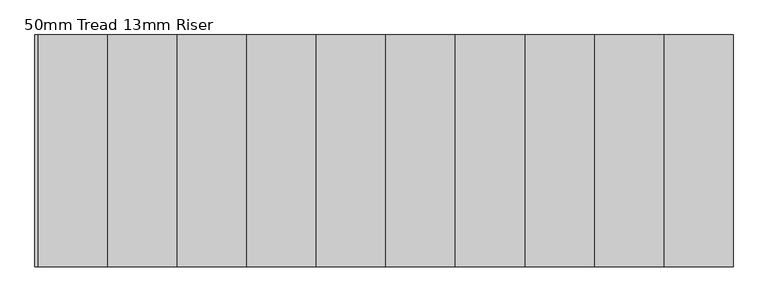
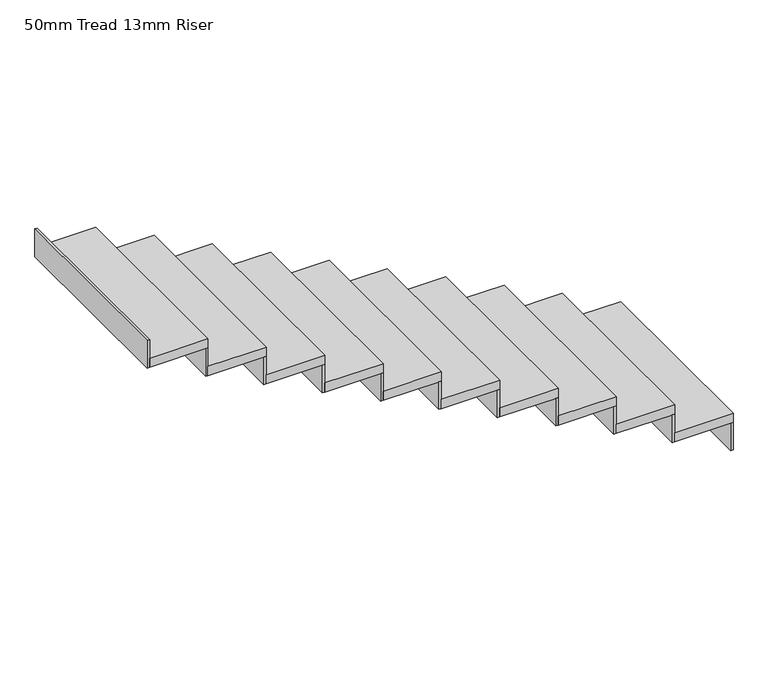
"""IFC4 building model written with IfcOpenShell, lengths in millimetres: stair flight geometry, 50mm Tread 13mm Riser."""

from ifc_helpers import new_model, si_unit, frame, origin, place, context, project, spatial, polyline, outline, extrude, source, transform, mapped, element, save


def stair_flight_50mm_tread_13mm_riser_afbce6aa(model_context):
    return source(origin(), model_context, "Body", "SweptSolid", [
        extrude(outline(polyline([(4676.3435815, -5376.491395), (4688.8435815, -5376.491395), (4688.8435815, -6376.491395), (4676.3435815, -6376.491395), (4676.3435815, -5376.491395)])), frame((0.0, 0.0, 1600.0), z_axis=(0.0, 0.0, 1.0), x_axis=(1.0, 0.0, 0.0)), (0.0, 0.0, 1.0), 150.0),
        extrude(outline(polyline([(4388.8435815, -6376.491395), (4388.8435815, -5376.491395), (4688.8435815, -5376.491395), (4688.8435815, -6376.491395), (4388.8435815, -6376.491395)])), frame((0.0, 0.0, 1750.0), z_axis=(0.0, 0.0, 1.0), x_axis=(1.0, 0.0, 0.0)), (0.0, 0.0, 1.0), 50.0),
        extrude(outline(polyline([(4376.3435815, -5376.491395), (4388.8435815, -5376.491395), (4388.8435815, -6376.491395), (4376.3435815, -6376.491395), (4376.3435815, -5376.491395)])), frame((0.0, 0.0, 1750.0), z_axis=(0.0, 0.0, 1.0), x_axis=(1.0, 0.0, 0.0)), (0.0, 0.0, 1.0), 150.0),
        extrude(outline(polyline([(4088.8435815, -6376.491395), (4088.8435815, -5376.491395), (4388.8435815, -5376.491395), (4388.8435815, -6376.491395), (4088.8435815, -6376.491395)])), frame((0.0, 0.0, 1900.0), z_axis=(0.0, 0.0, 1.0), x_axis=(1.0, 0.0, 0.0)), (0.0, 0.0, 1.0), 50.0),
        extrude(outline(polyline([(4076.3435815, -5376.491395), (4088.8435815, -5376.491395), (4088.8435815, -6376.491395), (4076.3435815, -6376.491395), (4076.3435815, -5376.491395)])), frame((0.0, 0.0, 1900.0), z_axis=(0.0, 0.0, 1.0), x_axis=(1.0, 0.0, 0.0)), (0.0, 0.0, 1.0), 150.0),
        extrude(outline(polyline([(3788.8435815, -6376.491395), (3788.8435815, -5376.491395), (4088.8435815, -5376.491395), (4088.8435815, -6376.491395), (3788.8435815, -6376.491395)])), frame((0.0, 0.0, 2050.0), z_axis=(0.0, 0.0, 1.0), x_axis=(1.0, 0.0, 0.0)), (0.0, 0.0, 1.0), 50.0),
        extrude(outline(polyline([(3776.3435815, -5376.491395), (3788.8435815, -5376.491395), (3788.8435815, -6376.491395), (3776.3435815, -6376.491395), (3776.3435815, -5376.491395)])), frame((0.0, 0.0, 2050.0), z_axis=(0.0, 0.0, 1.0), x_axis=(1.0, 0.0, 0.0)), (0.0, 0.0, 1.0), 150.0),
        extrude(outline(polyline([(3488.8435815, -6376.491395), (3488.8435815, -5376.491395), (3788.8435815, -5376.491395), (3788.8435815, -6376.491395), (3488.8435815, -6376.491395)])), frame((0.0, 0.0, 2200.0), z_axis=(0.0, 0.0, 1.0), x_axis=(1.0, 0.0, 0.0)), (0.0, 0.0, 1.0), 50.0),
        extrude(outline(polyline([(3476.3435815, -5376.491395), (3488.8435815, -5376.491395), (3488.8435815, -6376.491395), (3476.3435815, -6376.491395), (3476.3435815, -5376.491395)])), frame((0.0, 0.0, 2200.0), z_axis=(0.0, 0.0, 1.0), x_axis=(1.0, 0.0, 0.0)), (0.0, 0.0, 1.0), 150.0),
        extrude(outline(polyline([(3188.8435815, -6376.491395), (3188.8435815, -5376.491395), (3488.8435815, -5376.491395), (3488.8435815, -6376.491395), (3188.8435815, -6376.491395)])), frame((0.0, 0.0, 2350.0), z_axis=(0.0, 0.0, 1.0), x_axis=(1.0, 0.0, 0.0)), (0.0, 0.0, 1.0), 50.0),
        extrude(outline(polyline([(3176.3435815, -5376.491395), (3188.8435815, -5376.491395), (3188.8435815, -6376.491395), (3176.3435815, -6376.491395), (3176.3435815, -5376.491395)])), frame((0.0, 0.0, 2350.0), z_axis=(0.0, 0.0, 1.0), x_axis=(1.0, 0.0, 0.0)), (0.0, 0.0, 1.0), 150.0),
        extrude(outline(polyline([(2888.8435815, -6376.491395), (2888.8435815, -5376.491395), (3188.8435815, -5376.491395), (3188.8435815, -6376.491395), (2888.8435815, -6376.491395)])), frame((0.0, 0.0, 2500.0), z_axis=(0.0, 0.0, 1.0), x_axis=(1.0, 0.0, 0.0)), (0.0, 0.0, 1.0), 50.0),
        extrude(outline(polyline([(2876.3435815, -5376.491395), (2888.8435815, -5376.491395), (2888.8435815, -6376.491395), (2876.3435815, -6376.491395), (2876.3435815, -5376.491395)])), frame((0.0, 0.0, 2500.0), z_axis=(0.0, 0.0, 1.0), x_axis=(1.0, 0.0, 0.0)), (0.0, 0.0, 1.0), 150.0),
        extrude(outline(polyline([(2588.8435815, -6376.491395), (2588.8435815, -5376.491395), (2888.8435815, -5376.491395), (2888.8435815, -6376.491395), (2588.8435815, -6376.491395)])), frame((0.0, 0.0, 2650.0), z_axis=(0.0, 0.0, 1.0), x_axis=(1.0, 0.0, 0.0)), (0.0, 0.0, 1.0), 50.0),
        extrude(outline(polyline([(2576.3435815, -5376.491395), (2588.8435815, -5376.491395), (2588.8435815, -6376.491395), (2576.3435815, -6376.491395), (2576.3435815, -5376.491395)])), frame((0.0, 0.0, 2650.0), z_axis=(0.0, 0.0, 1.0), x_axis=(1.0, 0.0, 0.0)), (0.0, 0.0, 1.0), 150.0),
        extrude(outline(polyline([(2288.8435815, -6376.491395), (2288.8435815, -5376.491395), (2588.8435815, -5376.491395), (2588.8435815, -6376.491395), (2288.8435815, -6376.491395)])), frame((0.0, 0.0, 2800.0), z_axis=(0.0, 0.0, 1.0), x_axis=(1.0, 0.0, 0.0)), (0.0, 0.0, 1.0), 50.0),
        extrude(outline(polyline([(2276.3435815, -5376.491395), (2288.8435815, -5376.491395), (2288.8435815, -6376.491395), (2276.3435815, -6376.491395), (2276.3435815, -5376.491395)])), frame((0.0, 0.0, 2800.0), z_axis=(0.0, 0.0, 1.0), x_axis=(1.0, 0.0, 0.0)), (0.0, 0.0, 1.0), 150.0),
        extrude(outline(polyline([(1988.8435815, -6376.491395), (1988.8435815, -5376.491395), (2288.8435815, -5376.491395), (2288.8435815, -6376.491395), (1988.8435815, -6376.491395)])), frame((0.0, 0.0, 2950.0), z_axis=(0.0, 0.0, 1.0), x_axis=(1.0, 0.0, 0.0)), (0.0, 0.0, 1.0), 50.0),
        extrude(outline(polyline([(1976.3435815, -5376.491395), (1988.8435815, -5376.491395), (1988.8435815, -6376.491395), (1976.3435815, -6376.491395), (1976.3435815, -5376.491395)])), frame((0.0, 0.0, 2950.0), z_axis=(0.0, 0.0, 1.0), x_axis=(1.0, 0.0, 0.0)), (0.0, 0.0, 1.0), 150.0),
        extrude(outline(polyline([(1676.3435815, -5376.491395), (1688.8435815, -5376.491395), (1688.8435815, -6376.491395), (1676.3435815, -6376.491395), (1676.3435815, -5376.491395)])), frame((0.0, 0.0, 3100.0), z_axis=(0.0, 0.0, 1.0), x_axis=(1.0, 0.0, 0.0)), (0.0, 0.0, 1.0), 150.0),
        extrude(outline(polyline([(1688.8435815, -6376.491395), (1688.8435815, -5376.491395), (1988.8435815, -5376.491395), (1988.8435815, -6376.491395), (1688.8435815, -6376.491395)])), frame((0.0, 0.0, 3100.0), z_axis=(0.0, 0.0, 1.0), x_axis=(1.0, 0.0, 0.0)), (0.0, 0.0, 1.0), 50.0),
    ])


if __name__ == "__main__":
    model = new_model("IFC4")
    model_context = context("Model", 3, world=origin())
    ifc_project = project(units=[si_unit("LENGTHUNIT", "METRE", prefix="MILLI")], contexts=[model_context])
    site = spatial("IfcSite", under=ifc_project)
    building = spatial("IfcBuilding", under=site)
    placement = place(None, origin())
    stair_flight_50mm_tread_13mm_riser_shape = stair_flight_50mm_tread_13mm_riser_afbce6aa(model_context)
    element("IfcStairFlight", 1, ObjectType="50mm Tread 13mm Riser", at=placement, inside=building, context=model_context, shape_type="MappedRepresentation", body=[
        mapped(stair_flight_50mm_tread_13mm_riser_shape, transform((0.0, 0.0, 0.0), x_axis=(1.0, 0.0, 0.0), y_axis=(0.0, 1.0, 0.0), z_axis=(0.0, 0.0, 1.0))),
    ])
    save(model, "model.ifc")
